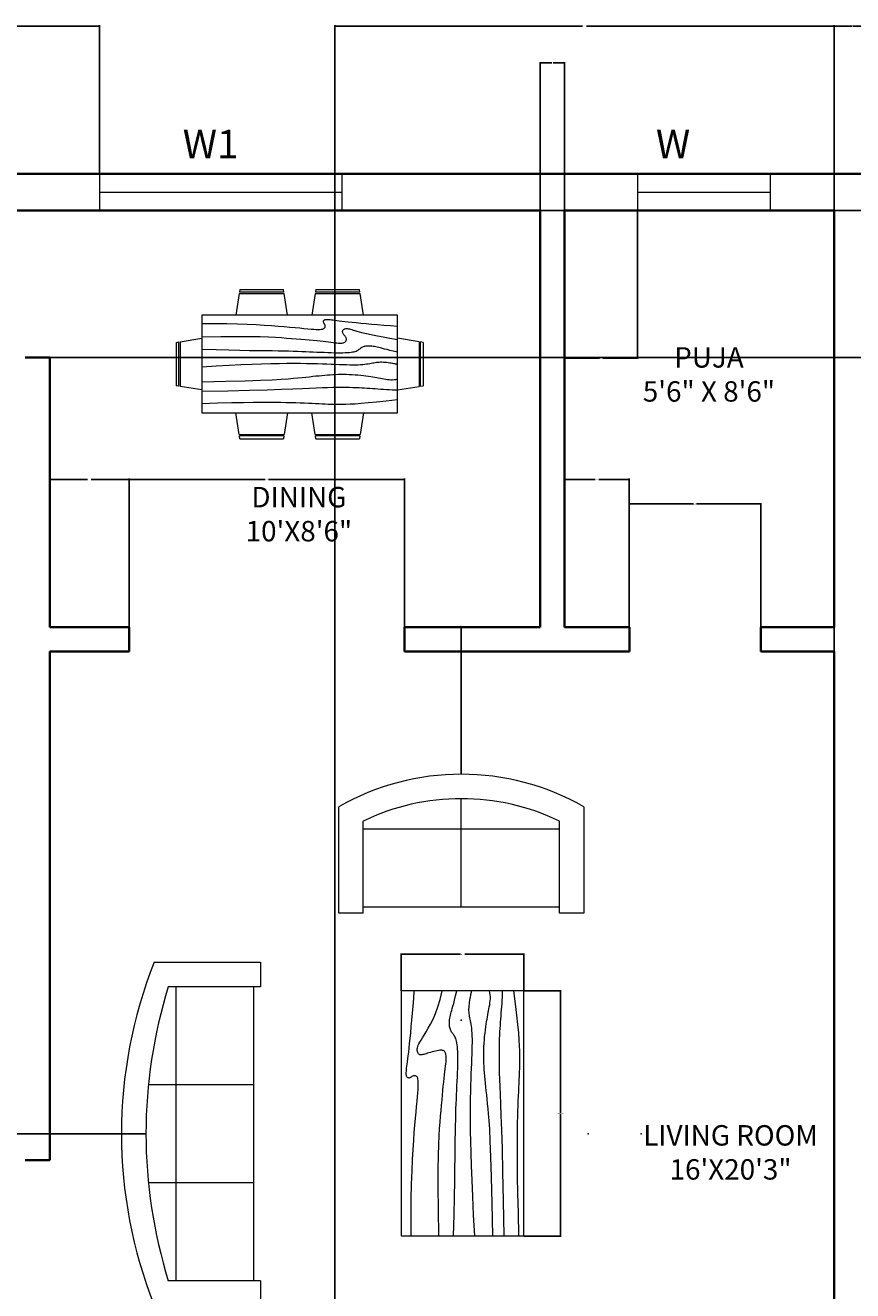
# Model space of a CAD drawing. Units: inches. Extents: x 1939 to 2674, y 558 to 1170.
# Tile 3 of 6: x 2104 to 2307, y 861 to 1170. Entities that reach past the tile are written whole.
import ezdxf

# ---------------------------------------------------------------- set-up
doc = ezdxf.new("R2010")
doc.units = ezdxf.units.IN
for name, color, linetype, lineweight in [('A-ANNO-DIMS', 2, 'Continuous', 18), ('A-ANNO-TEXT', 7, 'Continuous', 18), ('A-AREA-IDEN', 7, 'Continuous', 18), ('A-FURN', 8, 'Continuous', 13), ('A-GLAZ', 4, 'Continuous', 18), ('A-WALL', 7, 'Continuous', 35)]:
    doc.layers.add(name, color=color, linetype=linetype, lineweight=lineweight)
doc.styles.get("Standard").update_dxf_attribs({"font": 'arial.ttf'})
doc.dimstyles.get("Standard").update_dxf_attribs({"dimtxt": 0.18, "dimasz": 0.18, "dimexe": 0.18, "dimexo": 0.0625, "dimgap": 0.09, "dimtad": 0, "dimtih": 1, "dimtoh": 1, "dimdec": 4, "dimzin": 0, "dimdsep": 46, "dimtxsty": 'Standard', "dimcen": 0.09, "dimadec": 0, "dimazin": 0, "dimtfac": 1, "dimtdec": 4, "dimtofl": 0, "dimtmove": 0, "dimatfit": 3, "dimfxl": 1, "dimtolj": 1, "dimtzin": 0, "dimarcsym": 0})

# ---------------------------------------------------------------- blocks, each defined once
blk = doc.blocks.new('Dining Set - 36 x 72 in.')
for p, q in [((-22.2343, 26.00059), (-23.4847, 17.99762)), ((-22.2304, 26), (-5.7608, 26)), ((-22, 27.5), (-22.1562, 26.50042)), ((-5.8416, 26.5), (-22.1534, 26.5)), ((-22, 27.5), (-6, 27.5)), ((-5.8437, 26.49966), (-6, 27.5)), ((-4.5152, 17.99762), (-5.7655, 25.99926)), ((5.7657, 26.00059), (4.5153, 17.99762)), ((5.7696, 26), (22.2392, 26)), ((6, 27.5), (5.8438, 26.50042)), ((22.1584, 26.5), (5.8466, 26.5)), ((6, 27.5), (22, 27.5)), ((22.1563, 26.49966), (22, 27.5)), ((23.4848, 17.99762), (22.2345, 25.99926)), ((36, 18), (-36, 18)), ((-36, 18), (-36, -18)), ((36, -18), (36, 18)), ((-44.0006, 8.23428), (-35.9976, 9.48474)), ((44.0006, 8.23428), (35.9976, 9.48474)), ((-45.5, 8), (-44.5004, 8.15617)), ((-45.5, 8), (-45.5, -8)), ((-44.5, -8.15843), (-44.5, 8.15338)), ((-44, 8.23041), (-44, -8.23915)), ((44, 8.23041), (44, -8.23915)), ((44.5, -8.15843), (44.5, 8.15338)), ((45.5, 8), (44.5005, 8.15617)), ((45.5, 8), (45.5, -8)), ((-44.4997, -8.15631), (-45.5, -8)), ((-35.9976, -9.48476), (-43.9993, -8.2345)), ((35.9976, -9.48476), (43.9993, -8.2345)), ((44.4997, -8.15631), (45.5, -8)), ((-36, -18), (36, -18)), ((-22.2343, -26.0006), (-23.4847, -17.99762)), ((-4.5152, -17.99762), (-5.7655, -25.99928)), ((5.7657, -26.0006), (4.5153, -17.99762)), ((23.4848, -17.99762), (22.2345, -25.99928)), ((-22.2304, -26), (-5.7608, -26)), ((-22, -27.5), (-22.1562, -26.50044)), ((-5.8416, -26.5), (-22.1534, -26.5)), ((-22, -27.5), (-6, -27.5)), ((-5.8437, -26.49967), (-6, -27.5)), ((5.7696, -26), (22.2392, -26)), ((6, -27.5), (5.8438, -26.50044)), ((22.1584, -26.5), (5.8466, -26.5)), ((6, -27.5), (22, -27.5)), ((22.1563, -26.49967), (22, -27.5))]:
    blk.add_line(p, q)
for points in [[(-36, 15), (-31.1772, 14.97754), (-26.8079, 14.91406), (-22.8538, 14.81543), (-19.276, 14.6875), (-16.0362, 14.53613), (-13.0957, 14.36718), (-10.4159, 14.18652), (-7.9583, 14), (-5.6904, 13.81315), (-3.6035, 13.63021), (-1.6954, 13.45508), (0.0365, 13.29166), (1.5945, 13.14388), (2.9811, 13.01562), (4.1988, 12.9108), (5.25, 12.83333), (6.1393, 12.78613), (6.8802, 12.76823), (7.4883, 12.77767), (7.9792, 12.8125), (8.3685, 12.87077), (8.6719, 12.95052), (8.9049, 13.0498), (9.0833, 13.16666), (9.2205, 13.29899), (9.3216, 13.44401), (9.3895, 13.59879), (9.4271, 13.76041), (9.4373, 13.92594), (9.4232, 14.09245), (9.3875, 14.257), (9.3333, 14.41666), (9.2638, 14.56917), (9.1836, 14.71484), (9.0975, 14.85465), (9.0104, 14.98958), (8.9272, 15.1206), (8.8529, 15.2487), (8.7922, 15.37483), (8.75, 15.5), (8.7305, 15.62467), (8.7344, 15.74739), (8.7617, 15.86621), (8.8125, 15.97916), (8.8867, 16.08431), (8.9844, 16.17968), (9.1055, 16.26334), (9.25, 16.33333), (9.4189, 16.38802), (9.6172, 16.42708), (9.8506, 16.45052), (10.125, 16.45833), (10.4463, 16.45052), (10.8203, 16.42708), (11.2529, 16.38802), (11.75, 16.33333), (12.3184, 16.26318), (12.9694, 16.17838), (13.7151, 16.07991), (14.5677, 15.96875), (15.5395, 15.84586), (16.6426, 15.71224), (17.8893, 15.56884), (19.2917, 15.41666), (20.859, 15.25667), (22.5879, 15.08984), (24.4721, 14.91715), (26.5052, 14.73958), (28.6809, 14.5581), (30.9929, 14.3737), (33.4347, 14.18733), (36, 14)], [(-36, 10), (-28.9766, 10.14274), (-23.1725, 10.20442), (-18.4241, 10.19775), (-14.5677, 10.13541), (-11.4399, 10.03011), (-8.877, 9.89453), (-6.7154, 9.74137), (-4.7917, 9.58333), (-2.9698, 9.43082), (-1.2246, 9.28515), (0.4415, 9.14534), (2.026, 9.01041), (3.5266, 8.87939), (4.9408, 8.7513), (6.266, 8.62516), (7.5, 8.5), (8.6411, 8.37549), (9.6914, 8.2539), (10.6538, 8.13818), (11.5312, 8.03125), (12.3267, 7.93603), (13.043, 7.85547), (13.6831, 7.79248), (14.25, 7.75), (14.7471, 7.7303), (15.1797, 7.73307), (15.5537, 7.75732), (15.875, 7.80208), (16.1494, 7.86637), (16.3828, 7.94922), (16.5811, 8.04964), (16.75, 8.16666), (16.8944, 8.29915), (17.0143, 8.44531), (17.1089, 8.60319), (17.1771, 8.77083), (17.218, 8.94629), (17.2305, 9.1276), (17.2137, 9.31282), (17.1667, 9.5), (17.0895, 9.6875), (16.987, 9.875), (16.8649, 10.0625), (16.7292, 10.25), (16.5856, 10.4375), (16.4401, 10.625), (16.2985, 10.8125), (16.1667, 11), (16.05, 11.18733), (15.9518, 11.3737), (15.8752, 11.5581), (15.8229, 11.73958), (15.798, 11.91715), (15.8034, 12.08984), (15.842, 12.25667), (15.9167, 12.41666), (16.0295, 12.56836), (16.1784, 12.70833), (16.3605, 12.83268), (16.5729, 12.9375), (16.8127, 13.01888), (17.0768, 13.07291), (17.3625, 13.0957), (17.6667, 13.08333), (17.9894, 13.03312), (18.3418, 12.94726), (18.7382, 12.82918), (19.1927, 12.68229), (19.7195, 12.51001), (20.3327, 12.31575), (21.0465, 12.10294), (21.875, 11.875), (22.8357, 11.63354), (23.959, 11.37304), (25.2786, 11.08618), (26.8282, 10.76562), (28.6414, 10.40405), (30.752, 9.99414), (33.1936, 9.52856), (36, 9)], [(-36, 5.5), (-30.7157, 5.3348), (-26.069, 5.20963), (-21.9946, 5.11767), (-18.4271, 5.05208), (-15.3009, 5.00602), (-12.5508, 4.97265), (-10.1112, 4.94515), (-7.9167, 4.91666), (-5.909, 4.88167), (-4.0586, 4.83984), (-2.3429, 4.79215), (-0.7396, 4.73958), (0.7739, 4.6831), (2.22, 4.6237), (3.6213, 4.56233), (5, 4.5), (6.373, 4.43782), (7.7344, 4.3776), (9.0723, 4.32129), (10.375, 4.27083), (11.6309, 4.22819), (12.8281, 4.19531), (13.9551, 4.17415), (15, 4.16666), (15.954, 4.17448), (16.819, 4.19791), (17.6001, 4.23698), (18.3021, 4.29166), (18.9299, 4.36198), (19.4883, 4.44791), (19.9823, 4.54948), (20.4167, 4.66666), (20.7969, 4.79899), (21.1302, 4.94401), (21.4245, 5.09879), (21.6875, 5.26041), (21.9271, 5.42594), (22.1511, 5.59245), (22.3672, 5.757), (22.5834, 5.91666), (22.8065, 6.06868), (23.0404, 6.21093), (23.2879, 6.34147), (23.5521, 6.45833), (23.8358, 6.55957), (24.142, 6.64323), (24.4735, 6.70735), (24.8334, 6.75), (25.2235, 6.76969), (25.642, 6.76692), (26.0858, 6.74267), (26.5521, 6.69791), (27.0379, 6.63362), (27.5404, 6.55078), (28.0565, 6.45036), (28.5834, 6.33333), (29.1242, 6.19987), (29.7071, 6.04687), (30.3661, 5.87044), (31.1354, 5.66666), (32.0493, 5.43164), (33.142, 5.16146), (34.4475, 4.85221), (36, 4.5)], [(-36, -1), (-30.7915, -0.6591), (-26.0195, -0.38216), (-21.6519, -0.16284), (-17.6563, 0.00521), (-14.0005, 0.12833), (-10.6523, 0.21289), (-7.5796, 0.26522), (-4.75, 0.29166), (-2.134, 0.29793), (0.2878, 0.28711), (2.5317, 0.26163), (4.6146, 0.22396), (6.5529, 0.17651), (8.3633, 0.12174), (10.0623, 0.06209), (11.6667, 0), (13.1899, -0.06201), (14.6341, -0.1211), (15.9982, -0.17432), (17.2813, -0.21875), (18.4823, -0.25147), (19.6003, -0.26953), (20.6343, -0.27002), (21.5834, -0.25), (22.4481, -0.20768), (23.2357, -0.14584), (23.9549, -0.06836), (24.6146, 0.02083), (25.2235, 0.11784), (25.7904, 0.21875), (26.3241, 0.31966), (26.8334, 0.41666), (27.3265, 0.50618), (27.8099, 0.58593), (28.2894, 0.65397), (28.7709, 0.70833), (29.2601, 0.74707), (29.763, 0.76823), (30.2855, 0.76985), (30.8334, 0.75), (31.4088, 0.70784), (31.9994, 0.64713), (32.589, 0.57275), (33.1615, 0.48958), (33.7008, 0.4025), (34.1908, 0.3164), (34.6153, 0.23616), (34.9584, 0.16666), (35.2099, 0.11165), (35.3848, 0.07031), (35.504, 0.04069), (35.5886, 0.02083), (35.6594, 0.00879), (35.7377, 0.0026), (35.8442, 0.00032), (36, 0)], [(-36, -6.5), (-27.1843, -6.31267), (-20.084, -6.1263), (-14.469, -5.9419), (-10.1094, -5.76042), (-6.7752, -5.58285), (-4.2363, -5.41016), (-2.2629, -5.24333), (-0.625, -5.08334), (0.8708, -4.93099), (2.2715, -4.78646), (3.5872, -4.64974), (4.8281, -4.52084), (6.0046, -4.39974), (7.127, -4.28646), (8.2053, -4.18099), (9.25, -4.08334), (10.2705, -3.99382), (11.2734, -3.91407), (12.2647, -3.84603), (13.25, -3.79167), (14.2354, -3.75293), (15.2266, -3.73177), (16.2295, -3.73015), (17.25, -3.75), (18.2912, -3.79248), (19.3451, -3.85547), (20.4009, -3.93604), (21.4479, -4.03125), (22.4754, -4.13819), (23.4727, -4.25391), (24.4289, -4.37549), (25.3334, -4.5), (26.1785, -4.62492), (26.9694, -4.74935), (27.7145, -4.87281), (28.4219, -4.99479), (29.1, -5.11483), (29.7572, -5.23242), (30.4016, -5.34709), (31.0417, -5.45834), (31.6837, -5.56437), (32.3262, -5.65821), (32.9658, -5.73153), (33.599, -5.77604), (34.2224, -5.78345), (34.8327, -5.74545), (35.4264, -5.65373), (36, -5.5)], [(-36, -10), (-26.4022, -9.81299), (-18.4675, -9.62891), (-11.9839, -9.45069), (-6.7396, -9.28125), (-2.5226, -9.12354), (0.8789, -8.98047), (3.6769, -8.85498), (6.0833, -8.75), (8.2767, -8.66765), (10.3021, -8.60677), (12.1712, -8.56543), (13.8958, -8.54167), (15.4876, -8.53353), (16.9583, -8.53907), (18.3197, -8.55632), (19.5834, -8.58334), (20.7616, -8.61841), (21.8685, -8.66081), (22.9188, -8.71004), (23.9271, -8.76563), (24.9081, -8.82707), (25.8763, -8.89388), (26.8465, -8.96558), (27.8334, -9.04167), (28.8474, -9.12118), (29.8828, -9.20117), (30.93, -9.27824), (31.9792, -9.34896), (33.0205, -9.40991), (34.0443, -9.45768), (35.0407, -9.48885), (36, -9.5)], [(-36, -14.5), (-30.0881, -14.33513), (-25.0332, -14.21224), (-20.7312, -14.12647), (-17.0781, -14.07292), (-13.97, -14.04671), (-11.3027, -14.04297), (-8.9724, -14.05681), (-6.875, -14.08334), (-4.9224, -14.11833), (-3.0905, -14.16016), (-1.3709, -14.20785), (0.2448, -14.26042), (1.7647, -14.3169), (3.1973, -14.3763), (4.5507, -14.43767), (5.8333, -14.5), (7.0554, -14.5621), (8.235, -14.62175), (9.3922, -14.67652), (10.5469, -14.72396), (11.7192, -14.76164), (12.929, -14.78711), (14.1965, -14.79794), (15.5417, -14.79167), (16.9933, -14.76424), (18.6152, -14.70508), (20.4804, -14.60197), (22.6615, -14.44271), (25.2312, -14.21509), (28.2624, -13.9069), (31.8277, -13.50594), (36, -13)]]:
    blk.add_lwpolyline(points)
blk = doc.blocks.new('Sofa - Roundback 7 ft.')
for p, q in [((-12.00002, -32.4421), (-12.00003, -6.5971)), ((11.99997, -32.4421), (11.99998, -6.5971)), ((-36.000027, -34), (-36.000027, -11.4696)), ((35.99998, -34), (35.99998, -11.4696)), ((-35.999844, -13.3819), (35.9998, -13.3819)), ((-36.000027, -32.4421), (35.99998, -32.4421))]:
    blk.add_line(p, q)
for points in [[(-36.000027, -34), (-42.000027, -34), (-42.000027, -8)], [(41.99998, -8), (41.99998, -34), (35.99998, -34)]]:
    blk.add_lwpolyline(points)
for centre, radius, start, end in [((0, -114.25), 114.25, 68.43141, 111.5686), ((-0.00001, -127.1968), 121.1968, 72.72033, 107.2797)]:
    blk.add_arc(centre, radius, start, end)
blk = doc.blocks.new('Sofa - Roundback Loveseat 5 ft.')
for p, q in [((0, -32.44198), (0, -5.99998)), ((-24, -33.99998), (-24, -11.46958)), ((24.00004, -33.99998), (24.00004, -11.46958)), ((-23.9998, -13.38178), (23.99986, -13.38178)), ((-24, -32.44198), (24.00004, -32.44198))]:
    blk.add_line(p, q)
for points in [[(-24, -33.99998), (-30, -33.99998), (-30, -7.99998)], [(30.00004, -7.99998), (30.00004, -33.99998), (24.00004, -33.99998)]]:
    blk.add_lwpolyline(points)
for centre, radius, start, end in [((0, -60.24998), 60.24998, 60.13715, 119.8628), ((0, -61.38438), 55.38444, 64.32083, 115.6792)]:
    blk.add_arc(centre, radius, start, end)
blk = doc.blocks.new('Table - Rectangular Woodgrain 60 x 30 in.')
for p, q in [((0, 0), (0, -30)), ((60, 0), (0, 0)), ((60, -30), (60, 0)), ((0, -30), (60, -30))]:
    blk.add_line(p, q)
for points in [[(0, -2.4), (4.8155, -2.418), (9.0302, -2.4688), (12.709, -2.5477), (15.9167, -2.65), (18.7181, -2.7711), (21.1781, -2.9063), (23.3616, -3.0508), (25.3333, -3.2), (27.1477, -3.3495), (28.8172, -3.4958), (30.3437, -3.636), (31.7291, -3.7667), (32.9756, -3.8849), (34.0849, -3.9875), (35.059, -4.0714), (35.9, -4.1334), (36.6114, -4.1711), (37.2041, -4.1854), (37.6906, -4.1779), (38.0833, -4.15), (38.3948, -4.1034), (38.6375, -4.0396), (38.8239, -3.9602), (38.9666, -3.8667), (39.0764, -3.7608), (39.1573, -3.6448), (39.2116, -3.521), (39.2416, -3.3917), (39.2498, -3.2593), (39.2385, -3.1261), (39.21, -2.9944), (39.1666, -2.8667), (39.111, -2.7447), (39.0468, -2.6281), (38.978, -2.5163), (38.9083, -2.4083), (38.8418, -2.3035), (38.7823, -2.201), (38.7337, -2.1001), (38.7, -2), (38.6844, -1.9003), (38.6875, -1.8021), (38.7094, -1.707), (38.75, -1.6167), (38.8094, -1.5326), (38.8875, -1.4563), (38.9844, -1.3893), (39.1, -1.3333), (39.2351, -1.2896), (39.3937, -1.2583), (39.5804, -1.2396), (39.8, -1.2333), (40.057, -1.2396), (40.3562, -1.2583), (40.7023, -1.2896), (41.1, -1.3333), (41.5547, -1.3895), (42.0755, -1.4573), (42.6721, -1.5361), (43.3542, -1.625), (44.1316, -1.7233), (45.014, -1.8302), (46.0114, -1.9449), (47.1333, -2.0667), (48.3862, -2.1947), (49.7625, -2.3281), (51.2513, -2.4663), (52.8416, -2.6083), (54.5226, -2.7535), (56.2833, -2.9011), (58.1127, -3.0501), (60, -3.2)], [(0, -9.2), (6.5759, -9.0858), (11.9385, -9.0365), (16.2527, -9.0418), (19.6833, -9.0917), (22.3952, -9.1759), (24.5531, -9.2844), (26.322, -9.4069), (27.8666, -9.5333), (29.3241, -9.6553), (30.7203, -9.7719), (32.0532, -9.8837), (33.3208, -9.9917), (34.5213, -10.0965), (35.6526, -10.199), (36.7128, -10.2999), (37.7, -10.4), (38.6129, -10.4996), (39.4531, -10.5969), (40.223, -10.6895), (40.925, -10.775), (41.5613, -10.8512), (42.1344, -10.9156), (42.6465, -10.966), (43.1, -11), (43.4976, -11.0158), (43.8437, -11.0136), (44.143, -10.9942), (44.4, -10.9583), (44.6195, -10.9069), (44.8062, -10.8406), (44.9648, -10.7603), (45.1, -10.6667), (45.2155, -10.5598), (45.3114, -10.4365), (45.3871, -10.2929), (45.4416, -10.125), (45.4743, -9.929), (45.4844, -9.7011), (45.4709, -9.4371), (45.4333, -9.1333), (45.3716, -8.7883), (45.2896, -8.4104), (45.1919, -8.0107), (45.0833, -7.6), (44.9685, -7.1893), (44.8521, -6.7896), (44.7388, -6.4117), (44.6333, -6.0667), (44.54, -5.7628), (44.4614, -5.4979), (44.4001, -5.2675), (44.3583, -5.0667), (44.3384, -4.8909), (44.3427, -4.7354), (44.3736, -4.5956), (44.4333, -4.4667), (44.5236, -4.3453), (44.6427, -4.2333), (44.7884, -4.1339), (44.9583, -4.05), (45.1501, -3.9849), (45.3614, -3.9417), (45.59, -3.9234), (45.8333, -3.9333), (46.0915, -3.9749), (46.3734, -4.0531), (46.6906, -4.1736), (47.0542, -4.3417), (47.4756, -4.5629), (47.9661, -4.8427), (48.5372, -5.1866), (49.2, -5.6), (49.9676, -6.0844), (50.8594, -6.625), (51.8965, -7.2031), (53.1, -7.8), (54.491, -8.3969), (56.0906, -8.975), (57.9199, -9.5156), (60, -10)], [(0, -12.8), (5.1847, -12.9322), (9.6213, -13.0323), (13.3963, -13.1059), (16.5958, -13.1583), (19.3063, -13.1952), (21.614, -13.2219), (23.6054, -13.2439), (25.3666, -13.2667), (26.9728, -13.2947), (28.4531, -13.3281), (29.8256, -13.3663), (31.1083, -13.4083), (32.3191, -13.4535), (33.476, -13.501), (34.597, -13.5501), (35.7, -13.6), (36.7984, -13.6497), (37.8875, -13.6979), (38.9578, -13.743), (40, -13.7833), (41.0047, -13.8174), (41.9625, -13.8438), (42.864, -13.8607), (43.7, -13.8667), (44.4631, -13.8604), (45.1552, -13.8417), (45.7801, -13.8104), (46.3416, -13.7667), (46.8439, -13.7104), (47.2906, -13.6417), (47.6858, -13.5604), (48.0333, -13.4667), (48.3375, -13.3608), (48.6042, -13.2448), (48.8396, -13.121), (49.05, -12.9917), (49.2417, -12.8593), (49.4208, -12.7261), (49.5937, -12.5944), (49.7667, -12.4667), (49.9452, -12.3451), (50.1323, -12.2313), (50.3303, -12.1268), (50.5416, -12.0333), (50.7686, -11.9524), (51.0135, -11.8854), (51.2788, -11.8341), (51.5666, -11.8), (51.8785, -11.7843), (52.2116, -11.7865), (52.562, -11.8059), (52.926, -11.8417), (53.2998, -11.8931), (53.6795, -11.9594), (54.0614, -12.0397), (54.4416, -12.1333), (54.8223, -12.2401), (55.2293, -12.3625), (55.6942, -12.5037), (56.2489, -12.6667), (56.9251, -12.8547), (57.7545, -13.0708), (58.7689, -13.3182), (60, -13.6)], [(0, -18), (5.124, -17.7273), (9.6609, -17.5057), (13.6705, -17.3303), (17.2125, -17.1958), (20.3467, -17.0973), (23.1328, -17.0297), (25.6307, -16.9878), (27.9, -16.9667), (29.9928, -16.9617), (31.9302, -16.9703), (33.7254, -16.9907), (35.3917, -17.0208), (36.9423, -17.0588), (38.3906, -17.1026), (39.7499, -17.1503), (41.0333, -17.2), (42.2519, -17.2496), (43.4073, -17.2969), (44.4986, -17.3395), (45.525, -17.375), (46.4858, -17.4012), (47.3802, -17.4156), (48.2074, -17.416), (48.9667, -17.4), (49.6583, -17.3662), (50.2872, -17.3167), (50.8595, -17.2547), (51.3812, -17.1833), (51.8584, -17.1057), (52.2971, -17.025), (52.7034, -16.9443), (53.0833, -16.8667), (53.443, -16.7951), (53.789, -16.7313), (54.128, -16.6768), (54.4666, -16.6334), (54.8115, -16.6024), (55.1693, -16.5854), (55.5465, -16.5841), (55.95, -16.6), (56.3828, -16.6337), (56.8346, -16.6823), (57.2915, -16.7418), (57.7396, -16.8084), (58.165, -16.878), (58.5539, -16.9469), (58.8924, -17.0111), (59.1666, -17.0667), (59.3679, -17.1107), (59.5078, -17.1438), (59.6032, -17.1675), (59.6708, -17.1833), (59.7275, -17.193), (59.7901, -17.1979), (59.8753, -17.1998), (60, -17.2)], [(0, -22.4), (8.0098, -22.2501), (14.4094, -22.1011), (19.4168, -21.9535), (23.25, -21.8083), (26.1269, -21.6663), (28.2656, -21.5281), (29.884, -21.3947), (31.2, -21.2667), (32.3967, -21.1448), (33.5172, -21.0292), (34.5697, -20.9198), (35.5625, -20.8167), (36.5037, -20.7198), (37.4015, -20.6292), (38.2642, -20.5448), (39.1, -20.4667), (39.9164, -20.3951), (40.7187, -20.3313), (41.5117, -20.2768), (42.3, -20.2333), (43.0883, -20.2024), (43.8812, -20.1854), (44.6836, -20.1841), (45.5, -20.2), (46.3328, -20.234), (47.1747, -20.2844), (48.0163, -20.3488), (48.8479, -20.425), (49.66, -20.5106), (50.4429, -20.6031), (51.1872, -20.7004), (51.8833, -20.8), (52.5246, -20.8999), (53.1166, -20.9995), (53.6681, -21.0983), (54.1875, -21.1958), (54.6834, -21.2919), (55.1646, -21.3859), (55.6394, -21.4777), (56.1167, -21.5667), (56.6028, -21.6515), (57.0961, -21.7266), (57.5929, -21.7852), (58.0896, -21.8208), (58.5823, -21.8268), (59.0674, -21.7964), (59.5412, -21.723), (60, -21.6)], [(0, -25.2), (8.6355, -25.0504), (15.7026, -24.9031), (21.4049, -24.7606), (25.9458, -24.625), (29.529, -24.4988), (32.3578, -24.3844), (34.6359, -24.284), (36.5667, -24.2), (38.3213, -24.1341), (39.9417, -24.0854), (41.437, -24.0523), (42.8167, -24.0333), (44.0901, -24.0268), (45.2667, -24.0313), (46.3557, -24.0451), (47.3667, -24.0667), (48.309, -24.0947), (49.1928, -24.1287), (50.0284, -24.168), (50.826, -24.2125), (51.5959, -24.2617), (52.3483, -24.3151), (53.0935, -24.3725), (53.8417, -24.4334), (54.6009, -24.497), (55.3699, -24.561), (56.1454, -24.6226), (56.9239, -24.6792), (57.7021, -24.7279), (58.4764, -24.7662), (59.2435, -24.7911), (60, -24.8)], [(0, -28.8), (5.6867, -28.6681), (10.45, -28.5698), (14.407, -28.5012), (17.675, -28.4584), (20.3711, -28.4374), (22.6125, -28.4344), (24.5164, -28.4455), (26.2, -28.4667), (27.762, -28.4947), (29.2276, -28.5281), (30.6033, -28.5663), (31.8958, -28.6084), (33.1118, -28.6535), (34.2578, -28.7011), (35.3405, -28.7501), (36.3666, -28.8), (37.3443, -28.8497), (38.288, -28.8974), (39.2137, -28.9412), (40.1375, -28.9792), (41.0753, -29.0093), (42.0432, -29.0297), (43.0572, -29.0384), (44.1333, -29.0333), (45.2936, -29.0114), (46.5843, -28.9641), (48.0579, -28.8816), (49.7666, -28.7542), (51.7629, -28.5721), (54.0989, -28.3255), (56.8272, -28.0048), (60, -27.6)]]:
    blk.add_lwpolyline(points)
blk = doc.blocks.new('WIN-PUJA')
for p, q in [((0, 9), (0, 0)), ((32.53, 0), (32.53, 9)), ((0, 4.5), (32.53, 4.5))]:
    blk.add_line(p, q)
blk = doc.blocks.new('WIN-DINING')
for p, q in [((0, 9), (0, 0)), ((59.38, 0), (59.38, 9)), ((0, 4.5), (59.38, 4.5))]:
    blk.add_line(p, q)
blk = doc.blocks.new('*D34')
at = {"layer": 'A-ANNO-DIMS', "color": 0, "lineweight": -2, "transparency": 16777216}
for p, q in [((2226.11, 934), (2235.23, 934)), ((2235.05, 933.82), (2235.05, 904.18)), ((2235.05, 874.18), (2235.05, 903.82)), ((2226.11, 874), (2235.23, 874))]:
    blk.add_line(p, q, dxfattribs=at)
at = {"layer": 'A-ANNO-DIMS', "color": 0, "transparency": 16777216}
for points in [[(2235.02, 933.82), (2235.08, 933.82), (2235.05, 934)], [(2235.02, 874.18), (2235.08, 874.18), (2235.05, 874)]]:
    blk.add_solid(points, dxfattribs=at)
at = {"layer": 'Defpoints', "color": 0, "transparency": 16777216}
for p in [(2226.05, 934), (2235.05, 934), (2226.05, 874)]:
    blk.add_point(p, dxfattribs=at)
at = {"layer": 'A-ANNO-DIMS', "color": 0, "transparency": 16777216, "insert": (2235.05, 904), "char_height": 0.18, "attachment_point": 5}
blk.add_mtext('\\A1;TABLE 60 TYP.', dxfattribs=at)
blk = doc.blocks.new('*D35')
at = {"layer": 'A-ANNO-DIMS', "color": 0, "lineweight": -2, "transparency": 16777216}
for p, q in [((2196.05, 934.07), (2196.05, 943.18)), ((2196.23, 943), (2210.52, 943)), ((2225.87, 943), (2211.58, 943)), ((2226.05, 934.07), (2226.05, 943.18))]:
    blk.add_line(p, q, dxfattribs=at)
at = {"layer": 'A-ANNO-DIMS', "color": 0, "transparency": 16777216}
for points in [[(2196.23, 943.03), (2196.23, 942.97), (2196.05, 943)], [(2225.87, 943.03), (2225.87, 942.97), (2226.05, 943)]]:
    blk.add_solid(points, dxfattribs=at)
at = {"layer": 'Defpoints', "color": 0, "transparency": 16777216}
for p in [(2196.05, 943), (2196.05, 934), (2226.05, 934)]:
    blk.add_point(p, dxfattribs=at)
at = {"layer": 'A-ANNO-DIMS', "color": 0, "transparency": 16777216, "insert": (2211.05, 943), "char_height": 0.18, "attachment_point": 5}
blk.add_mtext('\\A1;30 TYP.', dxfattribs=at)
blk = doc.blocks.new('*D56')
at = {"layer": 'A-ANNO-DIMS', "color": 0, "lineweight": -2, "transparency": 16777216}
for p, q in [((2129.44, 1023.17), (2129.44, 1059.44)), ((2129.62, 1059.26), (2162.76, 1059.26)), ((2196.68, 1059.26), (2163.55, 1059.26)), ((2196.86, 1023.17), (2196.86, 1059.44))]:
    blk.add_line(p, q, dxfattribs=at)
at = {"layer": 'A-ANNO-DIMS', "color": 0, "transparency": 16777216}
for points in [[(2129.62, 1059.29), (2129.62, 1059.23), (2129.44, 1059.26)], [(2196.68, 1059.29), (2196.68, 1059.23), (2196.86, 1059.26)]]:
    blk.add_solid(points, dxfattribs=at)
at = {"layer": 'Defpoints', "color": 0, "transparency": 16777216}
for p in [(2196.86, 1059.26), (2129.44, 1023.11), (2196.86, 1023.11)]:
    blk.add_point(p, dxfattribs=at)
at = {"layer": 'A-ANNO-DIMS', "color": 0, "transparency": 16777216, "insert": (2163.15, 1059.26), "char_height": 0.18, "attachment_point": 5}
blk.add_mtext('\\A1;67.42', dxfattribs=at)
blk = doc.blocks.new('*D57')
at = {"layer": 'A-ANNO-DIMS', "color": 0, "lineweight": -2, "transparency": 16777216}
for p, q in [((2251.88, 1017.17), (2251.88, 1053.44)), ((2284.03, 1017.17), (2284.03, 1053.44)), ((2252.06, 1053.26), (2267.56, 1053.26)), ((2283.85, 1053.26), (2268.35, 1053.26))]:
    blk.add_line(p, q, dxfattribs=at)
at = {"layer": 'A-ANNO-DIMS', "color": 0, "transparency": 16777216}
for points in [[(2252.06, 1053.29), (2252.06, 1053.23), (2251.88, 1053.26)], [(2283.85, 1053.29), (2283.85, 1053.23), (2284.03, 1053.26)]]:
    blk.add_solid(points, dxfattribs=at)
at = {"layer": 'Defpoints', "color": 0, "transparency": 16777216}
for p in [(2284.03, 1053.26), (2251.88, 1017.11), (2284.03, 1017.11)]:
    blk.add_point(p, dxfattribs=at)
at = {"layer": 'A-ANNO-DIMS', "color": 0, "transparency": 16777216, "insert": (2267.96, 1053.26), "char_height": 0.18, "attachment_point": 5}
blk.add_mtext('\\A1;32.15', dxfattribs=at)
blk = doc.blocks.new('*D58')
at = {"layer": 'A-ANNO-DIMS', "color": 0, "lineweight": -2, "transparency": 16777216}
for p, q in [((2179.79, 603.17), (2179.79, 1170.44)), ((2179.97, 1170.26), (2240.46, 1170.26)), ((2301.87, 1170.26), (2241.37, 1170.26)), ((2302.05, 594.17), (2302.05, 1170.44))]:
    blk.add_line(p, q, dxfattribs=at)
at = {"layer": 'A-ANNO-DIMS', "color": 0, "transparency": 16777216}
for points in [[(2179.97, 1170.29), (2179.97, 1170.23), (2179.79, 1170.26)], [(2301.87, 1170.29), (2301.87, 1170.23), (2302.05, 1170.26)]]:
    blk.add_solid(points, dxfattribs=at)
at = {"layer": 'Defpoints', "color": 0, "transparency": 16777216}
for p in [(2302.05, 1170.26), (2179.79, 603.11), (2302.05, 594.11)]:
    blk.add_point(p, dxfattribs=at)
at = {"layer": 'A-ANNO-DIMS', "color": 0, "transparency": 16777216, "insert": (2240.92, 1170.26), "char_height": 0.18, "attachment_point": 5}
blk.add_mtext('\\A1;122.26', dxfattribs=at)
blk = doc.blocks.new('*D59')
at = {"layer": 'A-ANNO-DIMS', "color": 0, "lineweight": -2, "transparency": 16777216}
for p, q in [((1975.05, 1134.17), (1975.05, 1170.44)), ((1975.23, 1170.26), (2048.18, 1170.26)), ((2122.04, 1170.26), (2049.09, 1170.26)), ((2122.22, 1134.17), (2122.22, 1170.44))]:
    blk.add_line(p, q, dxfattribs=at)
at = {"layer": 'A-ANNO-DIMS', "color": 0, "transparency": 16777216}
for points in [[(1975.23, 1170.29), (1975.23, 1170.23), (1975.05, 1170.26)], [(2122.04, 1170.29), (2122.04, 1170.23), (2122.22, 1170.26)]]:
    blk.add_solid(points, dxfattribs=at)
at = {"layer": 'Defpoints', "color": 0, "transparency": 16777216}
for p in [(2122.22, 1170.26), (1975.05, 1134.11), (2122.22, 1134.11)]:
    blk.add_point(p, dxfattribs=at)
at = {"layer": 'A-ANNO-DIMS', "color": 0, "transparency": 16777216, "insert": (2048.64, 1170.26), "char_height": 0.18, "attachment_point": 5}
blk.add_mtext('\\A1;147.18', dxfattribs=at)
blk = doc.blocks.new('*D60')
at = {"layer": 'A-ANNO-DIMS', "color": 0, "lineweight": -2, "transparency": 16777216}
for p, q in [((2236.05, 1125.05), (2236.05, 1088.78)), ((2253.9, 1125.05), (2253.9, 1088.78)), ((2236.23, 1088.96), (2244.59, 1088.96)), ((2253.72, 1088.96), (2245.36, 1088.96))]:
    blk.add_line(p, q, dxfattribs=at)
at = {"layer": 'A-ANNO-DIMS', "color": 0, "transparency": 16777216}
for points in [[(2236.23, 1088.99), (2236.23, 1088.93), (2236.05, 1088.96)], [(2253.72, 1088.99), (2253.72, 1088.93), (2253.9, 1088.96)]]:
    blk.add_solid(points, dxfattribs=at)
at = {"layer": 'Defpoints', "color": 0, "transparency": 16777216}
for p in [(2236.05, 1125.11), (2253.9, 1125.11), (2236.05, 1088.96)]:
    blk.add_point(p, dxfattribs=at)
at = {"layer": 'A-ANNO-DIMS', "color": 0, "transparency": 16777216, "insert": (2244.97, 1088.96), "char_height": 0.18, "attachment_point": 5}
blk.add_mtext('\\A1;17.85', dxfattribs=at)
blk = doc.blocks.new('*D65')
at = {"layer": 'A-ANNO-DIMS', "color": 0, "lineweight": -2, "transparency": 16777216}
for p, q in [((2122.29, 1125.11), (2674.38, 1125.11)), ((2674.2, 1124.93), (2674.2, 1107.29)), ((2674.2, 1089.29), (2674.2, 1106.93)), ((2104.11, 1089.11), (2674.38, 1089.11))]:
    blk.add_line(p, q, dxfattribs=at)
at = {"layer": 'A-ANNO-DIMS', "color": 0, "transparency": 16777216}
for points in [[(2674.17, 1124.93), (2674.23, 1124.93), (2674.2, 1125.11)], [(2674.17, 1089.29), (2674.23, 1089.29), (2674.2, 1089.11)]]:
    blk.add_solid(points, dxfattribs=at)
at = {"layer": 'Defpoints', "color": 0, "transparency": 16777216}
for p in [(2122.22, 1125.11), (2674.2, 1125.11), (2104.05, 1089.11)]:
    blk.add_point(p, dxfattribs=at)
at = {"layer": 'A-ANNO-DIMS', "color": 0, "transparency": 16777216, "insert": (2674.2, 1107.11), "char_height": 0.18, "attachment_point": 5}
blk.add_mtext('\\A1;36', dxfattribs=at)
blk = doc.blocks.new('*D68')
at = {"layer": 'A-ANNO-DIMS', "color": 0, "lineweight": -2, "transparency": 16777216}
for p, q in [((2230.05, 1125.17), (2230.05, 1161.44)), ((2230.23, 1161.26), (2232.9, 1161.26)), ((2235.87, 1161.26), (2233.2, 1161.26)), ((2236.05, 1125.17), (2236.05, 1161.44))]:
    blk.add_line(p, q, dxfattribs=at)
at = {"layer": 'A-ANNO-DIMS', "color": 0, "transparency": 16777216}
for points in [[(2230.23, 1161.29), (2230.23, 1161.23), (2230.05, 1161.26)], [(2235.87, 1161.29), (2235.87, 1161.23), (2236.05, 1161.26)]]:
    blk.add_solid(points, dxfattribs=at)
at = {"layer": 'Defpoints', "color": 0, "transparency": 16777216}
for p in [(2236.05, 1161.26), (2230.05, 1125.11), (2236.05, 1125.11)]:
    blk.add_point(p, dxfattribs=at)
at = {"layer": 'A-ANNO-DIMS', "color": 0, "transparency": 16777216, "insert": (2233.05, 1161.26), "char_height": 0.18, "attachment_point": 5}
blk.add_mtext('\\A1;6', dxfattribs=at)
blk = doc.blocks.new('*D70')
at = {"layer": 'A-ANNO-DIMS', "color": 0, "lineweight": -2, "transparency": 16777216}
for p, q in [((2302.05, 1125.17), (2302.05, 1170.44)), ((2302.23, 1170.26), (2306.4, 1170.26)), ((2310.87, 1170.26), (2306.7, 1170.26)), ((2311.05, 1125.17), (2311.05, 1170.44))]:
    blk.add_line(p, q, dxfattribs=at)
at = {"layer": 'A-ANNO-DIMS', "color": 0, "transparency": 16777216}
for points in [[(2302.23, 1170.29), (2302.23, 1170.23), (2302.05, 1170.26)], [(2310.87, 1170.29), (2310.87, 1170.23), (2311.05, 1170.26)]]:
    blk.add_solid(points, dxfattribs=at)
at = {"layer": 'Defpoints', "color": 0, "transparency": 16777216}
for p in [(2311.05, 1170.26), (2302.05, 1125.11), (2311.05, 1125.11)]:
    blk.add_point(p, dxfattribs=at)
at = {"layer": 'A-ANNO-DIMS', "color": 0, "transparency": 16777216, "insert": (2306.55, 1170.26), "char_height": 0.18, "attachment_point": 5}
blk.add_mtext('\\A1;9', dxfattribs=at)
blk = doc.blocks.new('*D71')
at = {"layer": 'A-ANNO-DIMS', "color": 0, "lineweight": -2, "transparency": 16777216}
for p, q in [((2110.05, 1023.17), (2110.05, 1059.44)), ((2110.23, 1059.26), (2119.29, 1059.26)), ((2129.26, 1059.26), (2120.2, 1059.26)), ((2129.44, 1023.17), (2129.44, 1059.44))]:
    blk.add_line(p, q, dxfattribs=at)
at = {"layer": 'A-ANNO-DIMS', "color": 0, "transparency": 16777216}
for points in [[(2110.23, 1059.29), (2110.23, 1059.23), (2110.05, 1059.26)], [(2129.26, 1059.29), (2129.26, 1059.23), (2129.44, 1059.26)]]:
    blk.add_solid(points, dxfattribs=at)
at = {"layer": 'Defpoints', "color": 0, "transparency": 16777216}
for p in [(2129.44, 1059.26), (2110.05, 1023.11), (2129.44, 1023.11)]:
    blk.add_point(p, dxfattribs=at)
at = {"layer": 'A-ANNO-DIMS', "color": 0, "transparency": 16777216, "insert": (2119.75, 1059.26), "char_height": 0.18, "attachment_point": 5}
blk.add_mtext('\\A1;19.396', dxfattribs=at)
blk = doc.blocks.new('*D72')
at = {"layer": 'A-ANNO-DIMS', "color": 0, "lineweight": -2, "transparency": 16777216}
for p, q in [((2236.05, 1023.17), (2236.05, 1059.44)), ((2236.23, 1059.26), (2243.51, 1059.26)), ((2251.7, 1059.26), (2244.42, 1059.26)), ((2251.88, 1023.17), (2251.88, 1059.44))]:
    blk.add_line(p, q, dxfattribs=at)
at = {"layer": 'A-ANNO-DIMS', "color": 0, "transparency": 16777216}
for points in [[(2236.23, 1059.29), (2236.23, 1059.23), (2236.05, 1059.26)], [(2251.7, 1059.29), (2251.7, 1059.23), (2251.88, 1059.26)]]:
    blk.add_solid(points, dxfattribs=at)
at = {"layer": 'Defpoints', "color": 0, "transparency": 16777216}
for p in [(2251.88, 1059.26), (2236.05, 1023.11), (2251.88, 1023.11)]:
    blk.add_point(p, dxfattribs=at)
at = {"layer": 'A-ANNO-DIMS', "color": 0, "transparency": 16777216, "insert": (2243.97, 1059.26), "char_height": 0.18, "attachment_point": 5}
blk.add_mtext('\\A1;15.835', dxfattribs=at)
blk = doc.blocks.new('*D73')
at = {"layer": 'A-ANNO-DIMS', "color": 0, "lineweight": -2, "transparency": 16777216}
for p, q in [((2061.53, 899.04), (2133.39, 899.04)), ((2254.68, 899.04), (2254.86, 899.04)), ((2254.77, 898.95), (2254.77, 899.13))]:
    blk.add_line(p, q, dxfattribs=at)
at = {"layer": 'A-ANNO-DIMS', "color": 0, "transparency": 16777216}
blk.add_solid([(2133.39, 899.07), (2133.39, 899.01), (2133.57, 899.04)], dxfattribs=at)
at = {"layer": 'Defpoints', "color": 0, "transparency": 16777216}
for p in [(2133.57, 899.04), (2254.77, 899.04)]:
    blk.add_point(p, dxfattribs=at)
at = {"layer": 'A-ANNO-DIMS', "color": 0, "transparency": 16777216, "insert": (2060.85, 899.04), "char_height": 0.18, "attachment_point": 5}
blk.add_mtext('\\A1;2X R121.2', dxfattribs=at)
blk = doc.blocks.new('*D74')
at = {"layer": 'A-ANNO-DIMS', "color": 0, "lineweight": -2, "transparency": 16777216}
for p, q in [((2059.77, 899.04), (2127.39, 899.04)), ((2241.73, 899.04), (2241.91, 899.04)), ((2241.82, 898.95), (2241.82, 899.13))]:
    blk.add_line(p, q, dxfattribs=at)
at = {"layer": 'A-ANNO-DIMS', "color": 0, "transparency": 16777216}
blk.add_solid([(2127.39, 899.07), (2127.39, 899.01), (2127.57, 899.04)], dxfattribs=at)
at = {"layer": 'Defpoints', "color": 0, "transparency": 16777216}
for p in [(2127.57, 899.04), (2241.82, 899.04)]:
    blk.add_point(p, dxfattribs=at)
at = {"layer": 'A-ANNO-DIMS', "color": 0, "transparency": 16777216, "insert": (2059.02, 899.04), "char_height": 0.18, "attachment_point": 5}
blk.add_mtext('\\A1;2X R114.25', dxfattribs=at)
blk = doc.blocks.new('*D75')
at = {"layer": 'A-ANNO-DIMS', "color": 0, "lineweight": -2, "transparency": 16777216}
for p, q in [((2210.58, 1023.22), (2210.76, 1023.22)), ((2210.76, 1023.22), (2210.76, 987.25)), ((2210.67, 926.82), (2210.85, 926.82)), ((2210.76, 926.73), (2210.76, 926.91))]:
    blk.add_line(p, q, dxfattribs=at)
at = {"layer": 'A-ANNO-DIMS', "color": 0, "transparency": 16777216}
blk.add_solid([(2210.79, 987.25), (2210.73, 987.25), (2210.76, 987.07)], dxfattribs=at)
at = {"layer": 'Defpoints', "color": 0, "transparency": 16777216}
for p in [(2210.76, 987.07), (2210.76, 926.82)]:
    blk.add_point(p, dxfattribs=at)
at = {"layer": 'A-ANNO-DIMS', "color": 0, "transparency": 16777216, "insert": (2209.9, 1023.22), "char_height": 0.18, "attachment_point": 5}
blk.add_mtext('\\A1;4X R60.25', dxfattribs=at)

msp = doc.modelspace()

# ---------------------------------------------------------------- linework, layer by layer
at = {"layer": 'A-WALL'}
for p, q in [((2638.048, 1134.1102), (1975.0479, 1134.1102)), ((1984.048, 1125.1102), (2230.048, 1125.1102)), ((2230.048, 1125.1102), (2230.048, 1023.1102)), ((2236.048, 1125.1102), (2236.048, 1023.1102)), ((2302.048, 1125.1102), (2236.048, 1125.1102)), ((2302.048, 1125.1102), (2302.048, 1023.1102)), ((2104.048, 1089.1102), (2110.048, 1089.1102)), ((2110.048, 1089.1102), (2110.048, 1023.1102)), ((2129.444, 1023.1102), (2110.048, 1023.1102)), ((2129.444, 1023.1102), (2129.444, 1017.1102)), ((2230.048, 1023.1102), (2196.8603, 1023.1102)), ((2196.8603, 1023.1102), (2196.8603, 1017.1102)), ((2251.8828, 1023.1102), (2236.048, 1023.1102)), ((2251.8828, 1023.1102), (2251.8828, 1017.1102)), ((2302.048, 1023.1102), (2284.0334, 1023.1102)), ((2284.0334, 1023.1102), (2284.0334, 1017.1102)), ((2129.444, 1017.1102), (2110.048, 1017.1102)), ((2110.048, 1017.1102), (2110.048, 892.6102)), ((2251.8828, 1017.1102), (2196.8603, 1017.1102)), ((2302.048, 1017.1102), (2284.0334, 1017.1102)), ((2302.048, 1017.1102), (2302.048, 771.1102)), ((2110.048, 892.6102), (2104.048, 892.6102))]:
    msp.add_line(p, q, dxfattribs=at)

# ---------------------------------------------------------------- block references
at = {"layer": 'A-FURN', "xscale": 0.6645132611138651, "yscale": 0.6645132611138651, "zscale": 0.6645132611138651}
msp.add_blockref('Dining Set - 36 x 72 in.', (2171.1929, 1087.4977), dxfattribs=at)
at = {"layer": 'A-FURN'}
msp.add_blockref('Sofa - Roundback Loveseat 5 ft.', (2210.7572, 987.0706), dxfattribs=at)
at = {"layer": 'A-FURN', "rotation": 90}
for name, p in [('Sofa - Roundback 7 ft.', (2127.5709, 899.043)), ('Table - Rectangular Woodgrain 60 x 30 in.', (2196.0498, 874.003))]:
    msp.add_blockref(name, p, dxfattribs=at)
at = {"layer": 'A-GLAZ'}
for name, p in [('WIN-DINING', (2122.2248, 1125.1102)), ('WIN-PUJA', (2253.8979, 1125.1102))]:
    msp.add_blockref(name, p, dxfattribs=at)

# ---------------------------------------------------------------- texts
at = {"layer": 'A-ANNO-TEXT', "char_height": 7, "attachment_point": 1}
for s, insert in [('\\pxqc;W1', (2138.4795, 1144.8586)), ('\\pxqc;W', (2251.6388, 1144.8586))]:
    msp.add_mtext_dynamic_manual_height_columns(s, width=21.893501, gutter_width=12.5, heights=[0], dxfattribs=dict(at, insert=insert))
at = {"layer": 'A-AREA-IDEN', "char_height": 5, "attachment_point": 1}
for s, width, insert in [('\\pxqc;PUJA\\P5\'6" X 8\'6"', 39.116177, (2251.8097, 1091.6289)), ('\\pxqc;DINING\\P10\'X8\'6"', 39.116177, (2151.4467, 1057.4144)), ('\\pxqc;LIVING ROOM\\P16\'X20\'3"', 49.102281, (2252.1091, 901.1429))]:
    msp.add_mtext_dynamic_manual_height_columns(s, width=width, gutter_width=12.5, heights=[0], dxfattribs=dict(at, insert=insert))

# ---------------------------------------------------------------- dimensions: what is measured, and where the dimension line sits
at = {"layer": 'A-ANNO-DIMS'}
for base, p1, p2, override, picture, middle in [((2122.2248, 1170.2602), (1975.0479, 1134.1102), (2122.2248, 1134.1102), {"dimdec": 2, "dimlfac": 1, "dimrnd": 0, "dimzin": 0, "dimdsep": 46, "dimlunit": 2}, '*D59', (2048.6364, 1170.2602)), ((2302.048, 1170.2602), (2179.7888, 603.1102), (2302.048, 594.1102), {"dimdec": 2, "dimlfac": 1, "dimrnd": 0, "dimzin": 0, "dimdsep": 46, "dimlunit": 2}, '*D58', (2240.9184, 1170.2602)), ((2311.048, 1170.2602), (2302.048, 1125.1102), (2311.048, 1125.1102), {"dimdec": 0, "dimlfac": 1, "dimrnd": 0, "dimzin": 0, "dimdsep": 46, "dimlunit": 2}, '*D70', (2306.548, 1170.2602)), ((2236.048, 1161.2602), (2230.048, 1125.1102), (2236.048, 1125.1102), {"dimdec": 0, "dimlfac": 1, "dimrnd": 0, "dimzin": 0, "dimdsep": 46, "dimlunit": 2}, '*D68', (2233.048, 1161.2602)), ((2129.444, 1059.2602), (2110.048, 1023.1102), (2129.444, 1023.1102), {"dimdec": 3, "dimlfac": 1, "dimrnd": 0, "dimzin": 0, "dimdsep": 46, "dimlunit": 2}, '*D71', (2119.746, 1059.2602)), ((2196.8603, 1059.2602), (2129.444, 1023.1102), (2196.8603, 1023.1102), {"dimdec": 2, "dimlfac": 1, "dimrnd": 0, "dimzin": 0, "dimdsep": 46, "dimlunit": 2}, '*D56', (2163.1521, 1059.2602)), ((2251.8828, 1059.2602), (2236.048, 1023.1102), (2251.8828, 1023.1102), {"dimdec": 3, "dimlfac": 1, "dimrnd": 0, "dimzin": 0, "dimdsep": 46, "dimlunit": 2}, '*D72', (2243.9654, 1059.2602)), ((2284.0334, 1053.2602), (2251.8828, 1017.1102), (2284.0334, 1017.1102), {"dimdec": 2, "dimlfac": 1, "dimrnd": 0, "dimzin": 0, "dimdsep": 46, "dimlunit": 2}, '*D57', (2267.9581, 1053.2602))]:
    dim = msp.add_linear_dim(base=base, p1=p1, p2=p2, dimstyle='Standard', override=override, dxfattribs=at)
    dim.commit()
    dim.dimension.update_dxf_attribs({"geometry": picture, "text_midpoint": middle})
for base, p1, p2, angle, override, picture, middle in [((2674.198, 1125.1102), (2104.048, 1089.1102), (2122.2248, 1125.1102), 90, {"dimdec": 0, "dimlfac": 1, "dimrnd": 0, "dimzin": 0, "dimdsep": 46, "dimlunit": 2}, '*D65', (2674.198, 1107.1102)), ((2236.048, 1088.9602), (2253.8979, 1125.1102), (2236.048, 1125.1102), 180, {"dimdec": 2, "dimlfac": 1, "dimrnd": 0, "dimzin": 0, "dimdsep": 46, "dimlunit": 2}, '*D60', (2244.9729, 1088.9602))]:
    dim = msp.add_linear_dim(base=base, p1=p1, p2=p2, angle=angle, dimstyle='Standard', override=override, dxfattribs=at)
    dim.commit()
    dim.dimension.update_dxf_attribs({"geometry": picture, "text_midpoint": middle})
for center, mpoint, text, override, picture, middle in [((2210.7572, 926.8207), (2210.757, 987.0706), '4X <>', {"dimdec": 2, "dimlfac": 1, "dimrnd": 0, "dimzin": 0, "dimdsep": 46, "dimlunit": 2}, '*D75', (2209.8993, 1023.2206)), ((2241.8209, 899.043), (2127.5709, 899.043), '2X <>', {"dimdec": 2, "dimlfac": 1, "dimrnd": 0, "dimzin": 0, "dimdsep": 46, "dimlunit": 2}, '*D74', (2059.0209, 899.043)), ((2254.7677, 899.043), (2133.5709, 899.043), '2X <>', {"dimdec": 1, "dimlfac": 1, "dimrnd": 0, "dimzin": 0, "dimdsep": 46, "dimlunit": 2}, '*D73', (2060.8528, 899.043))]:
    dim = msp.add_radius_dim(center=center, mpoint=mpoint, text=text, dimstyle='Standard', override=override, dxfattribs=at)
    dim.commit()
    dim.dimension.update_dxf_attribs({"geometry": picture, "text_midpoint": middle, "dimtype": 164})
for base, p1, p2, angle, text, picture, middle in [((2196.0498, 943.003), (2226.0498, 934.003), (2196.0498, 934.003), 180, '<> TYP.', '*D35', (2211.0498, 943.003)), ((2235.0498, 934.003), (2226.0498, 874.003), (2226.0498, 934.003), 90, 'TABLE <> TYP.', '*D34', (2235.0498, 904.003))]:
    dim = msp.add_linear_dim(base=base, p1=p1, p2=p2, angle=angle, text=text, dimstyle='Standard', override={"dimdec": 0, "dimlfac": 1, "dimrnd": 0, "dimzin": 0, "dimdsep": 46, "dimlunit": 2}, dxfattribs=at)
    dim.commit()
    dim.dimension.update_dxf_attribs({"geometry": picture, "text_midpoint": middle})

doc.saveas('drawing.dxf')
